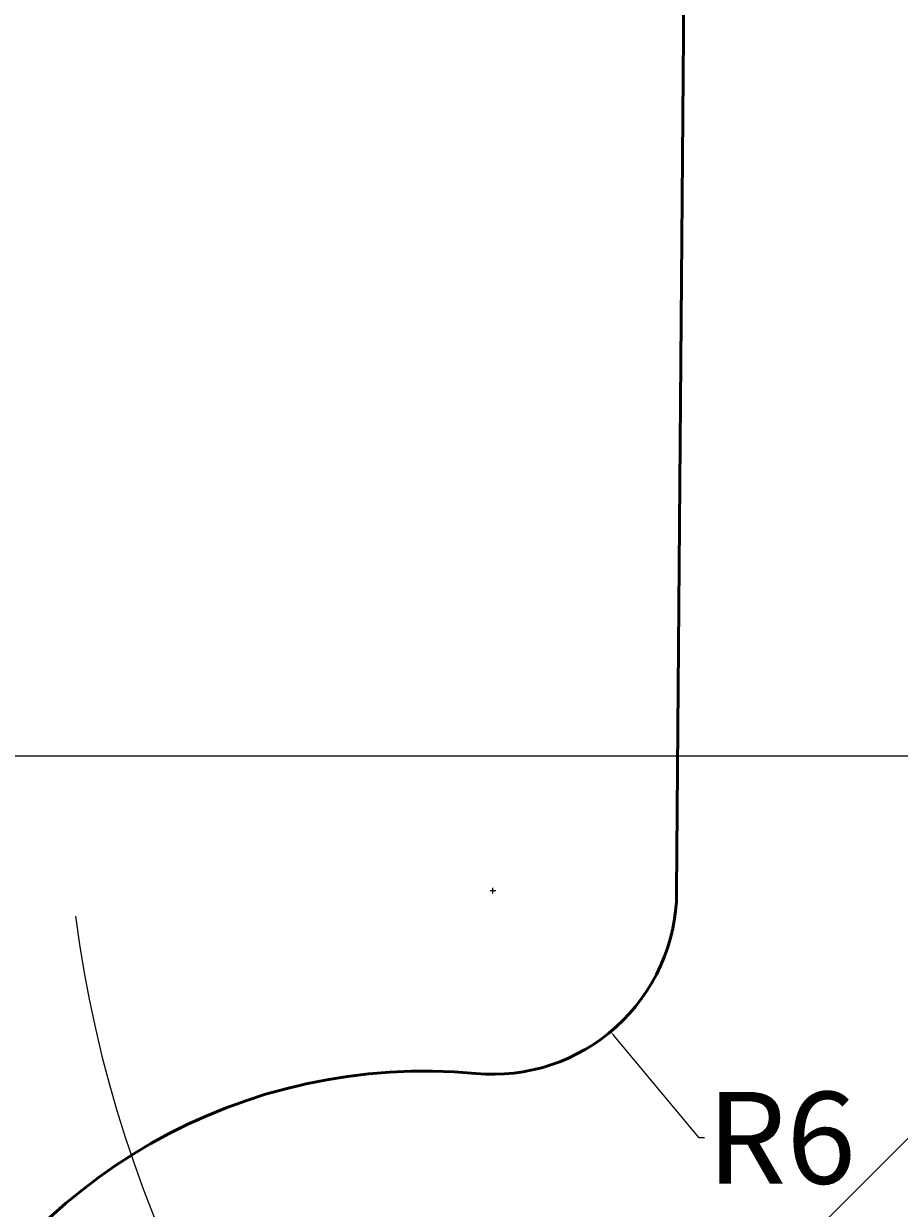
# Model space of a CAD drawing. Units: millimetres. Extents: x -53 to 92, y -147 to 37.
# Tile 6 of 16: x -22 to 6, y -69 to -30. Entities that reach past the tile are written whole.
import ezdxf

# ---------------------------------------------------------------- set-up
doc = ezdxf.new("R2010")
doc.units = ezdxf.units.MM
doc.header["$MEASUREMENT"] = 0
doc.linetypes.add('CENTER', pattern=[50.8, 31.75, -6.35, 6.35, -6.35])
for name, color, linetype, lineweight in [('M-CNTR', 4, 'CENTER', 18), ('M-DIMS', 2, 'Continuous', 25), ('M-OUTL', 7, 'Continuous', 50)]:
    doc.layers.add(name, color=color, linetype=linetype, lineweight=lineweight)
doc.styles.get("Standard").update_dxf_attribs({"font": 'arial.ttf'})
doc.dimstyles.get("Standard").update_dxf_attribs({"dimtxt": 0.18, "dimasz": 0.18, "dimexe": 0.18, "dimexo": 0.0625, "dimgap": 0.09, "dimtad": 0, "dimtih": 1, "dimtoh": 1, "dimdec": 4, "dimzin": 0, "dimdsep": 46, "dimtxsty": 'Standard', "dimcen": 0.09, "dimadec": 0, "dimazin": 0, "dimtfac": 1, "dimtdec": 4, "dimtofl": 0, "dimtmove": 0, "dimatfit": 3, "dimfxl": 1, "dimtolj": 1, "dimtzin": 0, "dimarcsym": 0})

# ---------------------------------------------------------------- blocks, each defined once
blk = doc.blocks.new('*D7')
at = {"layer": 'Defpoints', "color": 0, "transparency": 16777216}
for p in [(9.445, -3.88), (-44.321, -53.98), (18.956, -53.98)]:
    blk.add_point(p, dxfattribs=at)
at = {"layer": 'M-DIMS', "color": 0, "lineweight": -2, "transparency": 16777216}
for p, q in [((9.382, -3.88), (-44.501, -3.88)), ((-44.321, -4.06), (-44.321, -27.308)), ((-44.321, -53.8), (-44.321, -30.552)), ((18.894, -53.98), (-44.501, -53.98))]:
    blk.add_line(p, q, dxfattribs=at)
at = {"layer": 'M-DIMS', "color": 0, "transparency": 16777216}
for points in [[(-44.351, -4.06), (-44.291, -4.06), (-44.321, -3.88)], [(-44.351, -53.8), (-44.291, -53.8), (-44.321, -53.98)]]:
    blk.add_solid(points, dxfattribs=at)
at = {"layer": 'M-DIMS', "color": 0, "transparency": 16777216, "insert": (-44.321, -28.93), "char_height": 0.18, "attachment_point": 5}
blk.add_mtext('\\A1;{\\H16.66667x;50}', dxfattribs=at)
blk = doc.blocks.new('*D9')
at = {"layer": 'Defpoints', "color": 0, "transparency": 16777216}
for p in [(-7.079, -58.37), (-3.237, -62.978)]:
    blk.add_point(p, dxfattribs=at)
at = {"layer": 'M-DIMS', "color": 0, "lineweight": -2, "transparency": 16777216}
for p, q in [((-7.169, -58.37), (-6.989, -58.37)), ((-7.079, -58.46), (-7.079, -58.28)), ((-0.347, -66.445), (-3.122, -63.117)), ((-0.167, -66.445), (-0.347, -66.445))]:
    blk.add_line(p, q, dxfattribs=at)
at = {"layer": 'M-DIMS', "color": 0, "transparency": 16777216}
blk.add_solid([(-3.099, -63.097), (-3.145, -63.136), (-3.237, -62.978)], dxfattribs=at)
at = {"layer": 'M-DIMS', "color": 0, "transparency": 16777216, "insert": (2.341, -66.445), "char_height": 0.18, "attachment_point": 5}
blk.add_mtext('\\A1;{\\H16.66667x;R6}', dxfattribs=at)
blk = doc.blocks.new('*D10')
at = {"layer": 'Defpoints', "color": 0, "transparency": 16777216}
for p in [(64.593, -18.184), (-26.68, -89.776)]:
    blk.add_point(p, dxfattribs=at)
at = {"layer": 'M-DIMS', "color": 0, "lineweight": -2, "transparency": 16777216}
for p, q in [((77.384, -8.151), (64.734, -18.073)), ((77.564, -8.151), (77.384, -8.151)), ((18.866, -53.98), (19.046, -53.98)), ((18.956, -54.07), (18.956, -53.89))]:
    blk.add_line(p, q, dxfattribs=at)
at = {"layer": 'M-DIMS', "color": 0, "transparency": 16777216}
blk.add_solid([(64.716, -18.05), (64.753, -18.097), (64.593, -18.184)], dxfattribs=at)
at = {"layer": 'M-DIMS', "color": 0, "transparency": 16777216, "insert": (82.599, -8.151), "char_height": 0.18, "attachment_point": 5}
blk.add_mtext('\\A1;{\\H16.66667x;%%C116}', dxfattribs=at)
blk = doc.blocks.new('*D17')
at = {"layer": 'Defpoints', "color": 0, "transparency": 16777216}
for p in [(-46.81, 25.909), (28.564, 25.909), (18.165, -111.975)]:
    blk.add_point(p, dxfattribs=at)
at = {"layer": 'M-DIMS', "color": 0, "lineweight": -2, "transparency": 16777216}
for p, q in [((28.502, 25.909), (-46.99, 25.909)), ((-46.81, 25.729), (-46.81, -42.851)), ((-46.81, -111.795), (-46.81, -43.215)), ((18.102, -111.975), (-46.99, -111.975))]:
    blk.add_line(p, q, dxfattribs=at)
at = {"layer": 'M-DIMS', "color": 0, "transparency": 16777216}
for points in [[(-46.84, 25.729), (-46.78, 25.729), (-46.81, 25.909)], [(-46.84, -111.795), (-46.78, -111.795), (-46.81, -111.975)]]:
    blk.add_solid(points, dxfattribs=at)
at = {"layer": 'M-DIMS', "color": 0, "transparency": 16777216, "insert": (-46.81, -43.033), "char_height": 0.18, "attachment_point": 5}
blk.add_mtext('\\A1;137.88', dxfattribs=at)
blk = doc.blocks.new('*D24')
at = {"layer": 'Defpoints', "color": 0, "transparency": 16777216}
for p in [(18.956, -53.969), (2.002, -101.015)]:
    blk.add_point(p, dxfattribs=at)
at = {"layer": 'M-DIMS', "color": 0, "lineweight": -2, "transparency": 16777216}
for p, q in [((18.866, -53.969), (19.046, -53.969)), ((18.956, -54.059), (18.956, -53.879)), ((-8.171, -129.243), (1.941, -101.184)), ((-8.351, -129.243), (-8.171, -129.243))]:
    blk.add_line(p, q, dxfattribs=at)
at = {"layer": 'M-DIMS', "color": 0, "transparency": 16777216}
blk.add_solid([(1.912, -101.174), (1.969, -101.195), (2.002, -101.015)], dxfattribs=at)
at = {"layer": 'M-DIMS', "color": 0, "transparency": 16777216, "insert": (-8.813, -129.243), "char_height": 0.18, "attachment_point": 5}
blk.add_mtext('\\A1;R50.01', dxfattribs=at)

msp = doc.modelspace()

# ---------------------------------------------------------------- linework, layer by layer
at = {"layer": 'M-CNTR'}
msp.add_line((18.95638, -53.98007), (-27.00556, -99.94201), dxfattribs=at)
msp.add_arc((18.95638, -54.07007), 40, 187.365915, 352.627832, dxfattribs=at)
at = {"layer": 'M-OUTL'}
msp.add_line((-1.07952, -58.41764), (-0.64538, -3.86515), dxfattribs=at)
for centre, radius, start, end in [((18.95638, -53.98007), 58, 108.3895553, 70.0459142), ((-7.07933, -58.36989), 6, 264.624123, 359.54403), ((-9.32787, -82.26433), 18, 84.624123, 224.999991)]:
    msp.add_arc(centre, radius, start, end, dxfattribs=at)

# ---------------------------------------------------------------- dimensions: what is measured, and where the dimension line sits
at = {"layer": 'M-DIMS'}
dim = msp.add_linear_dim(base=(-46.8103, 25.90924), p1=(18.16452, -111.97467), p2=(28.56407, 25.90924), angle=90, dimstyle='Standard', override={"dimdec": 2, "dimlfac": 1, "dimrnd": 0, "dimzin": 0, "dimdsep": 46, "dimlunit": 2}, dxfattribs=at)
dim.commit()
dim.dimension.update_dxf_attribs({"geometry": '*D17', "text_midpoint": (-46.8103, -43.03271)})
dim = msp.add_linear_dim(base=(-44.32095, -53.98007), p1=(9.44461, -3.87977), p2=(18.95638, -53.98007), angle=90, text='{\\H16.66667x;50}', dimstyle='Standard', override={"dimclrd": 0, "dimclre": 0, "dimclrt": 0}, dxfattribs=at)
dim.commit()
dim.dimension.update_dxf_attribs({"geometry": '*D7', "text_midpoint": (-44.32095, -28.92992)})
dim = msp.add_diameter_dim_2p(p1=(-26.67986, -89.77579), p2=(64.59262, -18.18435), text='{\\H16.66667x;%%C116}', dimstyle='Standard', override={"dimclrd": 0, "dimclre": 0, "dimclrt": 0}, dxfattribs=at)
dim.commit()
dim.dimension.update_dxf_attribs({"geometry": '*D10', "text_midpoint": (82.59889, -8.15132), "dimtype": 163})
dim = msp.add_radius_dim(center=(18.95621, -53.96903), mpoint=(2.00175, -101.01516), dimstyle='Standard', override={"dimdec": 2, "dimlfac": 1, "dimrnd": 0, "dimzin": 0, "dimdsep": 46, "dimlunit": 2}, dxfattribs=at)
dim.commit()
dim.dimension.update_dxf_attribs({"geometry": '*D24', "text_midpoint": (-8.8134, -129.24283), "dimtype": 164})
dim = msp.add_radius_dim(center=(-7.07933, -58.36989), mpoint=(-3.23721, -62.97837), text='{\\H16.66667x;R6}', dimstyle='Standard', override={"dimclrd": 0, "dimclre": 0, "dimclrt": 0}, dxfattribs=at)
dim.commit()
dim.dimension.update_dxf_attribs({"geometry": '*D9', "text_midpoint": (2.34109, -66.44541), "dimtype": 164})

doc.saveas('drawing.dxf')
